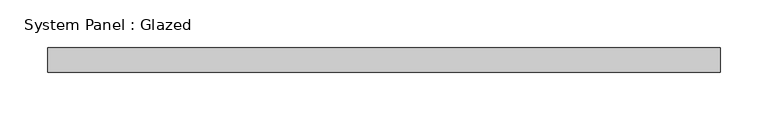
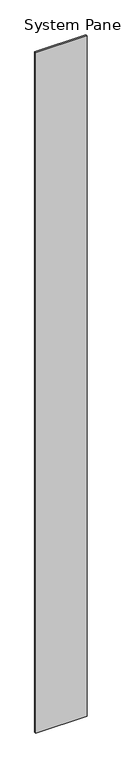
"""IFC4 building model written with IfcOpenShell, lengths in millimetres: plate geometry, System Panel : Glazed."""

from ifc_helpers import new_model, si_unit, origin, origin_with_axes, place, context, project, spatial, polyline, outline, extrude, source, transform, mapped, element, save


def system_panel_glazed_05561604(model_context):
    return source(origin(), model_context, "Body", "SweptSolid", [
        extrude(outline(polyline([(351.0490934, 19.05), (-351.0490934, 19.05), (-351.0490934, 44.45), (351.0490934, 44.45), (351.0490934, 19.05)])), origin_with_axes(), (0.0, 0.0, 1.0), 9863.981559),
    ])


if __name__ == "__main__":
    model = new_model("IFC4")
    model_context = context("Model", 3, world=origin())
    ifc_project = project(units=[si_unit("LENGTHUNIT", "METRE", prefix="MILLI")], contexts=[model_context])
    site = spatial("IfcSite", under=ifc_project)
    building = spatial("IfcBuilding", under=site)
    placement = place(None, origin())
    system_panel_glazed_shape = system_panel_glazed_05561604(model_context)
    element("IfcPlate", 1, ObjectType="System Panel : Glazed", at=placement, inside=building, context=model_context, shape_type="MappedRepresentation", body=[
        mapped(system_panel_glazed_shape, transform((0.0, 0.0, 0.0), x_axis=(1.0, 0.0, 0.0), y_axis=(0.0, 1.0, 0.0), z_axis=(0.0, 0.0, 1.0))),
    ])
    save(model, "model.ifc")

# Revit data of these elements
# Type "System Panel : Glazed"
#   Construction Type Id = "GSP4R"
#   Analytic Construction = "1/8 in Pilkington single glazing"
#   Visual Light Transmittance = 0.9
#   Solar Heat Gain Coefficient = 0.86
#   Heat Transfer Coefficient (U) = 1.18115 BTU/(h·ft²·°F)
# Element 1 (IfcPlate, "System Panel : Glazed")
#   Materials on its faces: "Glass"
# Materials
#   "Glass": class "Glass", colour RGB 0 128 192, transparency 0.75, Description = "Soda Lime Glass", Cost = 0
